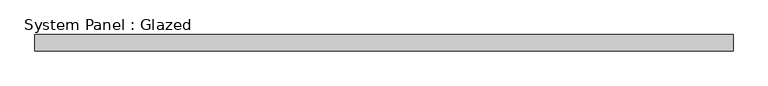
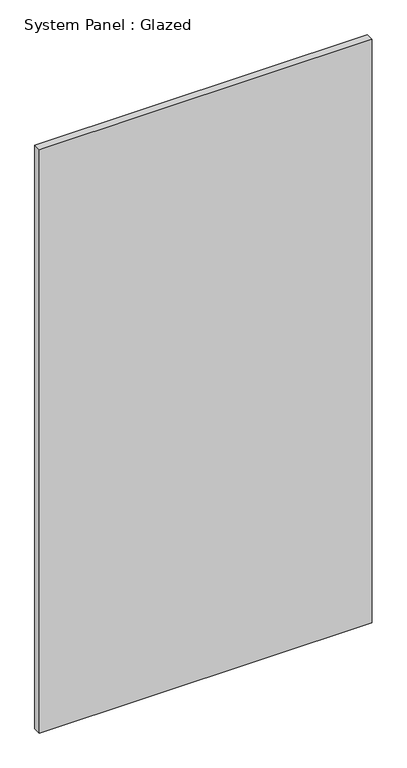
"""IFC4 building model written with IfcOpenShell, lengths in millimetres: plate geometry, System Panel : Glazed."""

from ifc_helpers import new_model, si_unit, origin, origin_with_axes, place, context, project, spatial, polyline, outline, extrude, source, transform, mapped, element, save


def system_panel_glazed_4fbe648e(model_context):
    return source(origin(), model_context, "Body", "SweptSolid", [
        extrude(outline(polyline([(549.2750001, 19.05), (-549.2750001, 19.05), (-549.2750001, 44.45), (549.2750001, 44.45), (549.2750001, 19.05)])), origin_with_axes(), (0.0, 0.0, 1.0), 2034.4673659),
    ])


if __name__ == "__main__":
    model = new_model("IFC4")
    model_context = context("Model", 3, world=origin())
    ifc_project = project(units=[si_unit("LENGTHUNIT", "METRE", prefix="MILLI")], contexts=[model_context])
    site = spatial("IfcSite", under=ifc_project)
    building = spatial("IfcBuilding", under=site)
    placement = place(None, origin())
    system_panel_glazed_shape = system_panel_glazed_4fbe648e(model_context)
    element("IfcPlate", 1, ObjectType="System Panel : Glazed", at=placement, inside=building, context=model_context, shape_type="MappedRepresentation", body=[
        mapped(system_panel_glazed_shape, transform((0.0, 0.0, 0.0), x_axis=(1.0, 0.0, 0.0), y_axis=(0.0, 1.0, 0.0), z_axis=(0.0, 0.0, 1.0))),
    ])
    save(model, "model.ifc")

# Revit data of these elements
# Type "System Panel : Glazed"
#   Construction Type Id = "GSP4R"
#   Analytic Construction = "1/8 in Pilkington single glazing"
#   Visual Light Transmittance = 0.9
#   Solar Heat Gain Coefficient = 0.86
#   Heat Transfer Coefficient (U) = 1.18115 BTU/(h·ft²·°F)
#   Define Thermal Properties by = 1
# Element 1 (IfcPlate, "System Panel : Glazed")
#   Materials on its faces: "glass panel 223"
# Materials
#   "glass panel 223": class "Generic", colour RGB 120 120 120, transparency 0, Cost = 0
